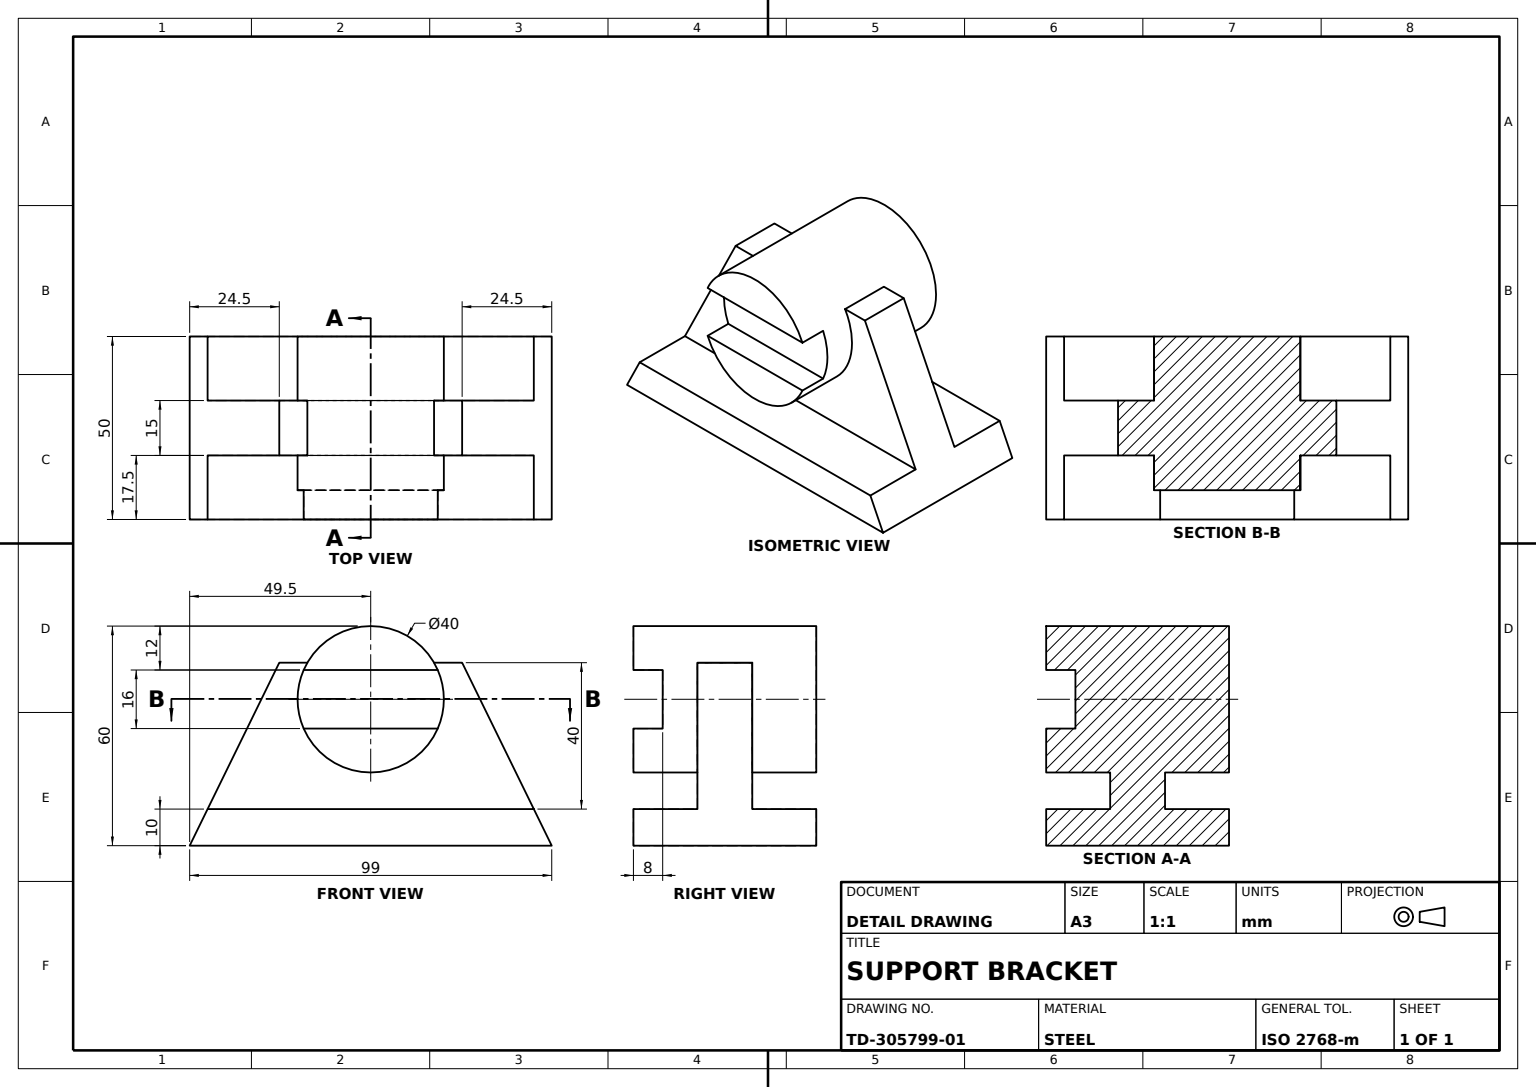
from build123d import *

# Parameters (mm, degrees)
BASE_PLATE_SKETCH_W     = 99
BASE_PLATE_SKETCH_H     = 50
BASE_PLATE_DEPTH        = 10
SUPPORT_BLOCK_SKETCH_W  = 99
SUPPORT_BLOCK_SKETCH_H  = 15
SUPPORT_BLOCK_DEPTH     = 40
SUPPORT_TAPER_CUT_DEPTH = 40
CYLINDER_BOSS_SKETCH_R  = 20
CYLINDER_BOSS_40_DEPTH  = 25
END_SLOT_SKETCH_W       = 47.327731092
END_SLOT_SKETCH_H       = 16
END_SLOT_16X8_DEPTH     = 8


with BuildPart() as part:
    # Base Plate Sketch → Base Plate (new body)
    with BuildSketch(Plane(origin=(0, 0, 0), x_dir=(1, 0, 0), z_dir=(0, 1, 0))):
        Rectangle(BASE_PLATE_SKETCH_W, BASE_PLATE_SKETCH_H)
    extrude(amount=BASE_PLATE_DEPTH)

    # Support Block Sketch → Support Block (add)
    with BuildSketch(Plane(origin=(0, 10, 0), x_dir=(1, 0, 0), z_dir=(0, 1, 0))):
        Rectangle(SUPPORT_BLOCK_SKETCH_W, SUPPORT_BLOCK_SKETCH_H)
    extrude(amount=SUPPORT_BLOCK_DEPTH)

    # Support Taper Sketch → Support Taper Cut (cut, symmetric)
    with BuildSketch(Plane.XY):
        Polygon((-25, 50), (-49.5, 0), (-49.5, 50), align=None)
        Polygon((25, 50), (49.5, 0), (49.5, 50), align=None)
    extrude(amount=SUPPORT_TAPER_CUT_DEPTH, both=True, mode=Mode.SUBTRACT)

    # Cylinder Boss Sketch → Cylinder Boss Ø40 (add, symmetric)
    with BuildSketch(Plane.XY):
        with Locations((0, 40)):
            Circle(CYLINDER_BOSS_SKETCH_R)
    extrude(amount=CYLINDER_BOSS_40_DEPTH, both=True)

    # End Slot Sketch → End Slot 16x8 (cut)
    with BuildSketch(Plane.XY.offset(25)):
        with Locations((0, 40)):
            Rectangle(END_SLOT_SKETCH_W, END_SLOT_SKETCH_H)
    extrude(amount=-END_SLOT_16X8_DEPTH, mode=Mode.SUBTRACT)


solid = part.part
